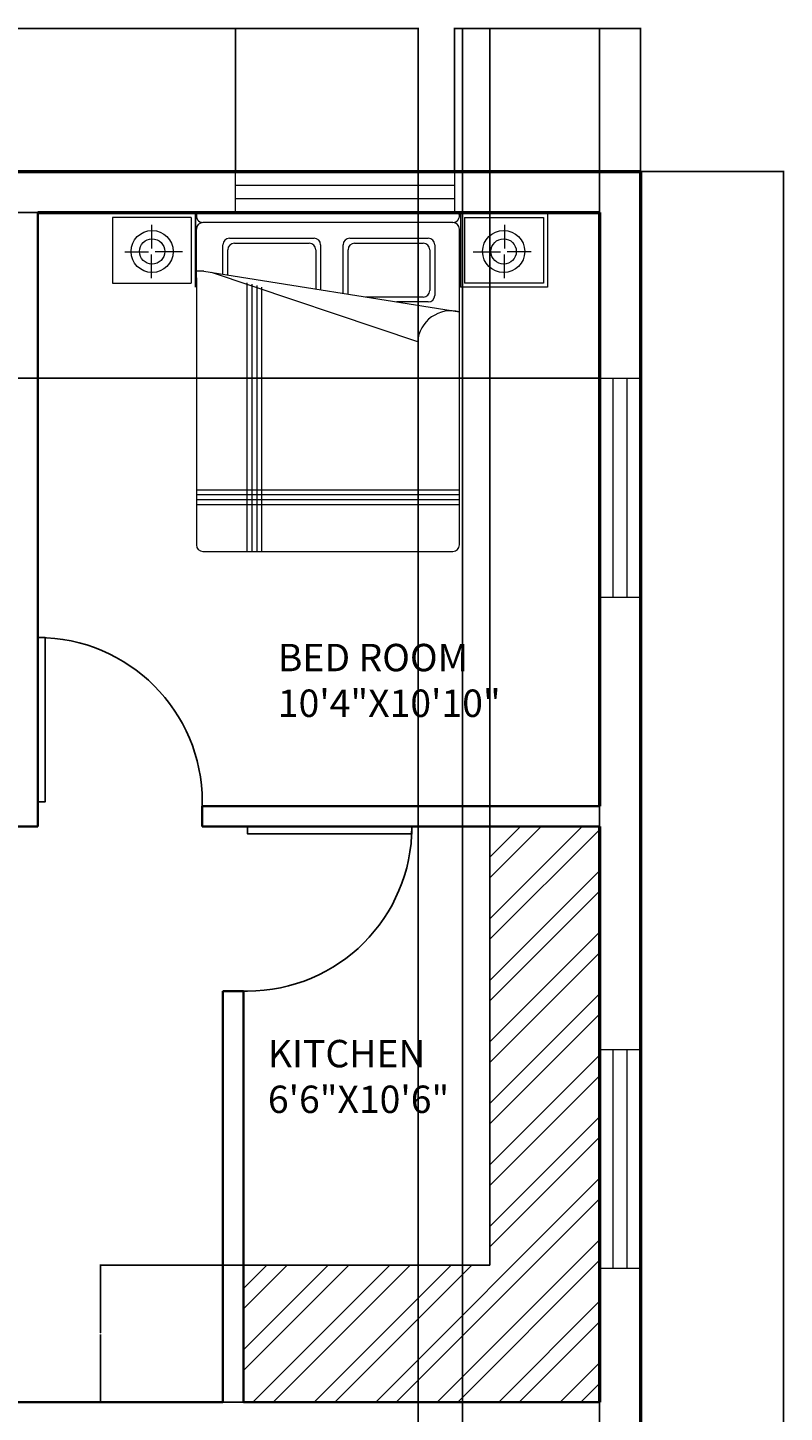
# Model space of a CAD drawing. Units: feet. Extents: x 2664 to 3060, y 1318 to 2005.
# Tile 5 of 5: x 2894 to 3060, y 1702 to 2005. Entities that reach past the tile are written whole.
import ezdxf

# ---------------------------------------------------------------- set-up
doc = ezdxf.new("R2010")
doc.units = ezdxf.units.FT
for name, color, linetype, lineweight in [('A-ANNO-DIMS', 2, 'Continuous', 18), ('A-AREA-IDEN', 109, 'Continuous', 18), ('A-WALL-EXTR', 130, 'Continuous', 50), ('DOOR', 249, 'Continuous', 25), ('FURNITURE', 240, 'Continuous', 13)]:
    doc.layers.add(name, color=color, linetype=linetype, lineweight=lineweight)
for name, color, linetype, lineweight, true_color in [('A-CASE', 41, 'Continuous', 25, 0xf5dd7a), ('A-CASE-PATT', 152, 'Continuous', 13, 0x2776bb), ('A-GLAZ', 222, 'Continuous', 18, 0xd4008b), ('A-WALL-INTR', 41, 'Continuous', 35, 0xf5dd7a)]:
    doc.layers.add(name, color=color, linetype=linetype, lineweight=lineweight, true_color=true_color)
doc.styles.get("Standard").update_dxf_attribs({"font": 'arial.ttf'})
doc.dimstyles.get("Standard").update_dxf_attribs({"dimtxt": 0.18, "dimasz": 0.18, "dimexe": 0.18, "dimexo": 0.0625, "dimgap": 0.09, "dimtad": 0, "dimtih": 1, "dimtoh": 1, "dimdec": 4, "dimzin": 0, "dimdsep": 46, "dimtxsty": 'Standard', "dimcen": 0.09, "dimadec": 0, "dimazin": 0, "dimtfac": 1, "dimtdec": 4, "dimtofl": 0, "dimtmove": 0, "dimatfit": 3, "dimfxl": 1, "dimtolj": 1, "dimtzin": 0, "dimarcsym": 0})

# ---------------------------------------------------------------- blocks, each defined once
blk = doc.blocks.new('*U2')
for p, q in [((0, 0), (0, -6)), ((40, 0), (40, -6))]:
    blk.add_line(p, q)
blk.add_lwpolyline([(0, 0), (0, 40), (1.75, 40), (1.75, 0)], close=True)
blk.add_arc((0, 0), 40, 0, 90)
blk = doc.blocks.new('BED-DOUBLE-WITH-NIGHTSTANDS')
for p, q in [((-29.54, 0), (-29.54, -16.21)), ((-30.37, -0.95), (-47.65, -0.95)), ((-47.65, -0.95), (-47.65, -15.35)), ((-39.11, -2.58), (-39.11, -7.74)), ((-30.37, -0.95), (-30.37, -15.35)), ((-29.47, -0.05), (-29.47, -16.25)), ((28.27, -0.11), (-29.17, -0.11)), ((26.92, -2.06), (-27.82, -2.06)), ((28.57, -0.05), (47.65, -0.05)), ((28.57, -0.05), (28.57, -16.25)), ((29.47, -0.95), (46.75, -0.95)), ((29.47, -0.95), (29.47, -15.35)), ((38.21, -2.58), (38.21, -7.74)), ((46.75, -0.95), (46.75, -15.35)), ((47.65, -0.05), (47.65, -16.25)), ((-29.26, -14.16), (-29.26, -3.5)), ((-22.01, -5.5), (-3.48, -5.5)), ((4.33, -5.5), (21.52, -5.5)), ((28.36, -72.65), (28.36, -3.5)), ((-44.95, -8.46), (-39.75, -8.46)), ((-39.11, -14.22), (-39.11, -9.06)), ((-32.27, -8.46), (-38.27, -8.46)), ((-23.45, -13.32), (-23.45, -6.94)), ((-22.37, -13.47), (-22.37, -8.02)), ((-20.93, -6.58), (-4.56, -6.58)), ((-3.12, -8.02), (-3.12, -16.63)), ((-2.04, -6.94), (-2.04, -16.8)), ((2.88, -17.58), (2.88, -6.94)), ((3.96, -17.76), (3.96, -8.02)), ((5.41, -6.58), (20.44, -6.58)), ((21.88, -8.02), (21.88, -16.94)), ((22.96, -6.94), (22.96, -18.02)), ((31.37, -8.46), (37.37, -8.46)), ((38.21, -14.22), (38.21, -9.06)), ((44.05, -8.46), (38.85, -8.46)), ((-27.62, -12.73), (-29.26, -12.73)), ((-29.26, -14.16), (-29.26, -72.65)), ((-27.62, -12.73), (28.36, -21.64)), ((-26, -12.96), (19.2, -28.15)), ((-47.65, -15.35), (-30.37, -15.35)), ((-18.14, -74.09), (-18.14, -15.24)), ((-17.06, -74.09), (-17.06, -15.55)), ((-15.97, -74.09), (-15.97, -15.86)), ((-14.89, -74.09), (-14.89, -16.18)), ((47.65, -16.25), (28.57, -16.25)), ((46.75, -15.35), (29.47, -15.35)), ((20.44, -18.38), (7.87, -18.38)), ((21.52, -19.46), (14.66, -19.46)), ((28.36, -60.64), (-29.26, -60.64)), ((28.36, -61.72), (-29.26, -61.72)), ((28.36, -62.8), (-29.26, -62.8)), ((28.36, -63.88), (-29.26, -63.88)), ((-27.82, -74.09), (26.92, -74.09))]:
    blk.add_line(p, q)
for centre, radius in [((-38.95, -8.4), 4.61), ((-38.95, -8.4), 2.77), ((38.05, -8.4), 4.61), ((38.05, -8.4), 2.77)]:
    blk.add_circle(centre, radius)
for centre, radius, start, end in [((-27.82, -0.62), 1.44, 159.2884, 270), ((-27.82, -3.5), 1.44, 90, 180), ((26.92, -0.62), 1.44, 270, 20.7116), ((26.92, -3.5), 1.44, 0, 90), ((-22.01, -6.94), 1.44, 90, 180), ((-3.48, -6.94), 1.44, 0, 90), ((4.33, -6.94), 1.44, 90, 180), ((21.52, -6.94), 1.44, 0, 90), ((-20.93, -8.02), 1.44, 90, 180), ((-4.56, -8.02), 1.44, 0, 90), ((5.41, -8.02), 1.44, 90, 180), ((20.44, -8.02), 1.44, 0, 90), ((20.44, -16.94), 1.44, 270, 0), ((21.52, -18.02), 1.44, 270, 0), ((26.5, -28.71), 7.32, 75.237, 175.5647), ((-27.82, -72.65), 1.44, 180, 270), ((26.92, -72.65), 1.44, 270, 0)]:
    blk.add_arc(centre, radius, start, end)
blk = doc.blocks.new('WINDOW-4FT')
for p, q in [((-24, 4.5), (24, 4.5)), ((-24, -4.5), (-24, 4.5)), ((24, 4.5), (24, -4.5)), ((-24, 1.5), (24, 1.5)), ((24, -1.5), (-24, -1.5)), ((24, -4.5), (-24, -4.5))]:
    blk.add_line(p, q)
blk = doc.blocks.new('*D33')
at = {"layer": 'A-ANNO-DIMS', "color": 0, "lineweight": -2, "transparency": 16777216}
for p, q in [((3028.34, 1973.57), (3059.74, 1973.57)), ((3059.56, 1973.39), (3059.56, 1661.75)), ((3059.56, 1349.75), (3059.56, 1661.39)), ((3028.34, 1349.57), (3059.74, 1349.57))]:
    blk.add_line(p, q, dxfattribs=at)
at = {"layer": 'A-ANNO-DIMS', "color": 0, "transparency": 16777216}
for points in [[(3059.53, 1973.39), (3059.59, 1973.39), (3059.56, 1973.57)], [(3059.53, 1349.75), (3059.59, 1349.75), (3059.56, 1349.57)]]:
    blk.add_solid(points, dxfattribs=at)
at = {"layer": 'Defpoints', "color": 0, "transparency": 16777216}
for p in [(3028.28, 1973.57), (3059.56, 1973.57), (3028.28, 1349.57)]:
    blk.add_point(p, dxfattribs=at)
at = {"layer": 'A-ANNO-DIMS', "color": 0, "transparency": 16777216, "insert": (3059.56, 1661.57), "char_height": 0.18, "attachment_point": 5}
blk.add_mtext('\\A1;624', dxfattribs=at)
blk = doc.blocks.new('*D38')
at = {"layer": 'A-ANNO-DIMS', "color": 0, "lineweight": -2, "transparency": 16777216}
for p, q in [((2875.93, 1973.63), (2875.93, 2005.03)), ((2876.11, 2004.85), (2907.35, 2004.85)), ((2939.35, 2004.85), (2908.11, 2004.85)), ((2939.53, 1973.63), (2939.53, 2005.03))]:
    blk.add_line(p, q, dxfattribs=at)
at = {"layer": 'A-ANNO-DIMS', "color": 0, "transparency": 16777216}
for points in [[(2876.11, 2004.88), (2876.11, 2004.82), (2875.93, 2004.85)], [(2939.35, 2004.88), (2939.35, 2004.82), (2939.53, 2004.85)]]:
    blk.add_solid(points, dxfattribs=at)
at = {"layer": 'Defpoints', "color": 0, "transparency": 16777216}
for p in [(2939.53, 2004.85), (2875.93, 1973.57), (2939.53, 1973.57)]:
    blk.add_point(p, dxfattribs=at)
at = {"layer": 'A-ANNO-DIMS', "color": 0, "transparency": 16777216, "insert": (2907.73, 2004.85), "char_height": 0.18, "attachment_point": 5}
blk.add_mtext('\\A1;63.61', dxfattribs=at)
blk = doc.blocks.new('*D39')
at = {"layer": 'A-ANNO-DIMS', "color": 0, "lineweight": -2, "transparency": 16777216}
for p, q in [((2987.53, 1973.63), (2987.53, 2005.03)), ((2987.71, 2004.85), (3007.51, 2004.85)), ((3028.1, 2004.85), (3008.31, 2004.85)), ((3028.28, 1973.63), (3028.28, 2005.03))]:
    blk.add_line(p, q, dxfattribs=at)
at = {"layer": 'A-ANNO-DIMS', "color": 0, "transparency": 16777216}
for points in [[(2987.71, 2004.88), (2987.71, 2004.82), (2987.53, 2004.85)], [(3028.1, 2004.88), (3028.1, 2004.82), (3028.28, 2004.85)]]:
    blk.add_solid(points, dxfattribs=at)
at = {"layer": 'Defpoints', "color": 0, "transparency": 16777216}
for p in [(3028.28, 2004.85), (2987.53, 1973.57), (3028.28, 1973.57)]:
    blk.add_point(p, dxfattribs=at)
at = {"layer": 'A-ANNO-DIMS', "color": 0, "transparency": 16777216, "insert": (3007.91, 2004.85), "char_height": 0.18, "attachment_point": 5}
blk.add_mtext('\\A1;40.75', dxfattribs=at)
blk = doc.blocks.new('*D47')
at = {"layer": 'A-ANNO-DIMS', "color": 0, "lineweight": -2, "transparency": 16777216}
for p, q in [((3019.22, 1964.57), (2663.82, 1964.57)), ((2664, 1964.39), (2664, 1946.59)), ((2664, 1928.43), (2664, 1946.23)), ((3019.22, 1928.25), (2663.82, 1928.25))]:
    blk.add_line(p, q, dxfattribs=at)
at = {"layer": 'A-ANNO-DIMS', "color": 0, "transparency": 16777216}
for points in [[(2663.97, 1964.39), (2664.03, 1964.39), (2664, 1964.57)], [(2663.97, 1928.43), (2664.03, 1928.43), (2664, 1928.25)]]:
    blk.add_solid(points, dxfattribs=at)
at = {"layer": 'Defpoints', "color": 0, "transparency": 16777216}
for p in [(3019.28, 1964.57), (2664, 1928.25), (3019.28, 1928.25)]:
    blk.add_point(p, dxfattribs=at)
at = {"layer": 'A-ANNO-DIMS', "color": 0, "transparency": 16777216, "insert": (2664, 1946.41), "char_height": 0.18, "attachment_point": 5}
blk.add_mtext('\\A1;36.32', dxfattribs=at)
blk = doc.blocks.new('*D48')
at = {"layer": 'A-ANNO-DIMS', "color": 0, "lineweight": -2, "transparency": 16777216}
for p, q in [((2879.53, 1619.63), (2879.53, 2005.03)), ((2879.71, 2004.85), (2929.25, 2004.85)), ((2979.35, 2004.85), (2929.81, 2004.85)), ((2979.53, 1619.63), (2979.53, 2005.03))]:
    blk.add_line(p, q, dxfattribs=at)
at = {"layer": 'A-ANNO-DIMS', "color": 0, "transparency": 16777216}
for points in [[(2879.71, 2004.88), (2879.71, 2004.82), (2879.53, 2004.85)], [(2979.35, 2004.88), (2979.35, 2004.82), (2979.53, 2004.85)]]:
    blk.add_solid(points, dxfattribs=at)
at = {"layer": 'Defpoints', "color": 0, "transparency": 16777216}
for p in [(2979.53, 2004.85), (2879.53, 1619.57), (2979.53, 1619.57)]:
    blk.add_point(p, dxfattribs=at)
at = {"layer": 'A-ANNO-DIMS', "color": 0, "transparency": 16777216, "insert": (2929.53, 2004.85), "char_height": 0.18, "attachment_point": 5}
blk.add_mtext('\\A1;100', dxfattribs=at)
blk = doc.blocks.new('*D56')
at = {"layer": 'A-ANNO-DIMS', "color": 0, "lineweight": -2, "transparency": 16777216}
for p, q in [((2995.28, 1830.13), (2995.28, 2005.03)), ((2995.46, 2004.85), (3007.06, 2004.85)), ((3019.1, 2004.85), (3007.5, 2004.85)), ((3019.28, 1830.13), (3019.28, 2005.03))]:
    blk.add_line(p, q, dxfattribs=at)
at = {"layer": 'A-ANNO-DIMS', "color": 0, "transparency": 16777216}
for points in [[(2995.46, 2004.88), (2995.46, 2004.82), (2995.28, 2004.85)], [(3019.1, 2004.88), (3019.1, 2004.82), (3019.28, 2004.85)]]:
    blk.add_solid(points, dxfattribs=at)
at = {"layer": 'Defpoints', "color": 0, "transparency": 16777216}
for p in [(3019.28, 2004.85), (2995.28, 1830.07), (3019.28, 1830.07)]:
    blk.add_point(p, dxfattribs=at)
at = {"layer": 'A-ANNO-DIMS', "color": 0, "transparency": 16777216, "insert": (3007.28, 2004.85), "char_height": 0.18, "attachment_point": 5}
blk.add_mtext('\\A1;24', dxfattribs=at)
blk = doc.blocks.new('*D57')
at = {"layer": 'A-ANNO-DIMS', "color": 0, "lineweight": -2, "transparency": 16777216}
for p, q in [((2941.22, 1734.07), (2909.82, 1734.07)), ((2910, 1733.89), (2910, 1719.25)), ((2910, 1704.25), (2910, 1718.89)), ((2941.22, 1704.07), (2909.82, 1704.07))]:
    blk.add_line(p, q, dxfattribs=at)
at = {"layer": 'A-ANNO-DIMS', "color": 0, "transparency": 16777216}
for points in [[(2909.97, 1733.89), (2910.03, 1733.89), (2910, 1734.07)], [(2909.97, 1704.25), (2910.03, 1704.25), (2910, 1704.07)]]:
    blk.add_solid(points, dxfattribs=at)
at = {"layer": 'Defpoints', "color": 0, "transparency": 16777216}
for p in [(2910, 1734.07), (2941.28, 1734.07), (2941.28, 1704.07)]:
    blk.add_point(p, dxfattribs=at)
at = {"layer": 'A-ANNO-DIMS', "color": 0, "transparency": 16777216, "insert": (2910, 1719.07), "char_height": 0.18, "attachment_point": 5}
blk.add_mtext('\\A1;30', dxfattribs=at)
blk = doc.blocks.new('*D58')
at = {"layer": 'A-ANNO-DIMS', "color": 0, "lineweight": -2, "transparency": 16777216}
for p, q in [((2989.28, 1488.63), (2989.28, 2005.03)), ((2989.46, 2004.85), (3004.06, 2004.85)), ((3019.1, 2004.85), (3004.5, 2004.85)), ((3019.28, 1488.63), (3019.28, 2005.03))]:
    blk.add_line(p, q, dxfattribs=at)
at = {"layer": 'A-ANNO-DIMS', "color": 0, "transparency": 16777216}
for points in [[(2989.46, 2004.88), (2989.46, 2004.82), (2989.28, 2004.85)], [(3019.1, 2004.88), (3019.1, 2004.82), (3019.28, 2004.85)]]:
    blk.add_solid(points, dxfattribs=at)
at = {"layer": 'Defpoints', "color": 0, "transparency": 16777216}
for p in [(3019.28, 2004.85), (2989.28, 1488.57), (3019.28, 1488.57)]:
    blk.add_point(p, dxfattribs=at)
at = {"layer": 'A-ANNO-DIMS', "color": 0, "transparency": 16777216, "insert": (3004.28, 2004.85), "char_height": 0.18, "attachment_point": 5}
blk.add_mtext('\\A1;30', dxfattribs=at)

msp = doc.modelspace()

# ---------------------------------------------------------------- hatches: boundary and pattern name
at = {"layer": 'A-CASE-PATT'}
h = msp.add_hatch(dxfattribs=at)
h.set_pattern_fill('ANSI32', color=256)
h.paths.add_polyline_path([(3019.28, 1615.071), (2941.28, 1615.071), (2941.28, 1585.071), (2989.28, 1585.071), (2989.28, 1488.571), (3019.28, 1488.571)])
h.paths.add_polyline_path([(3019.28, 1830.071), (2995.28, 1830.071), (2995.28, 1734.071), (2941.28, 1734.071), (2941.28, 1704.071), (3019.28, 1704.071)])

# ---------------------------------------------------------------- linework, layer by layer
at = {"layer": 'A-CASE'}
for p in [(2995.28, 1830.071), (2941.28, 1734.071)]:
    msp.add_line(p, (2995.28, 1734.071), dxfattribs=at)
at = {"layer": 'A-WALL-EXTR'}
for p, q in [((2704.28, 1973.571), (3028.28, 1973.571)), ((3028.28, 1973.571), (3028.28, 1349.571)), ((2896.28, 1964.571), (3019.28, 1964.571)), ((3019.28, 1964.571), (3019.28, 1834.571)), ((3019.28, 1830.071), (3019.28, 1704.071))]:
    msp.add_line(p, q, dxfattribs=at)
at = {"layer": 'A-WALL-INTR'}
for p, q in [((2896.28, 1834.571), (2896.28, 1964.571)), ((2896.28, 1834.571), (2896.28, 1830.071)), ((2932.28, 1834.571), (3019.28, 1834.571)), ((2932.28, 1834.571), (2932.28, 1830.071)), ((2891.78, 1830.071), (2896.28, 1830.071)), ((2932.28, 1830.071), (2936.78, 1830.071)), ((2936.78, 1830.071), (2941.28, 1830.071)), ((2941.28, 1830.071), (3019.28, 1830.071)), ((2936.78, 1794.071), (2936.78, 1704.071)), ((2936.78, 1794.071), (2941.28, 1794.071)), ((2941.28, 1794.071), (2941.28, 1704.071)), ((2866.78, 1704.071), (2936.78, 1704.071)), ((2941.28, 1704.071), (3019.28, 1704.071))]:
    msp.add_line(p, q, dxfattribs=at)

# ---------------------------------------------------------------- block references
at = {"layer": 'A-GLAZ'}
for p, rotation in [((2963.534, 1969.071), 180), ((3023.78, 1904.253), 89.99999999999844), ((3023.78, 1757.306), 89.99999999999864)]:
    msp.add_blockref('WINDOW-4FT', p, dxfattribs=dict(at, rotation=rotation))
at = {"layer": 'DOOR', "xscale": 0.899999999999959, "yscale": 0.899999999999959, "zscale": 0.899999999999959}
msp.add_blockref('*U2', (2896.28, 1835.471), dxfattribs=at)
at = {"layer": 'DOOR', "xscale": 0.899999999999959, "yscale": 0.899999999999959, "zscale": 0.899999999999959, "rotation": 270}
msp.add_blockref('*U2', (2942.18, 1830.071), dxfattribs=at)
at = {"layer": 'FURNITURE'}
msp.add_blockref('BED-DOUBLE-WITH-NIGHTSTANDS', (2960.234, 1964.426), dxfattribs=at)

# ---------------------------------------------------------------- texts
at = {"layer": 'A-AREA-IDEN', "char_height": 6, "attachment_point": 1}
for s, width, insert in [('BED ROOM \\P10\'4"X10\'10"', 48.82765, (2948.825, 1870.1)), ('KITCHEN\\P6\'6"X10\'6"', 22.955, (2946.648, 1783.368))]:
    msp.add_mtext_dynamic_manual_height_columns(s, width=width, gutter_width=12.5, heights=[0], dxfattribs=dict(at, insert=insert))

# ---------------------------------------------------------------- dimensions: what is measured, and where the dimension line sits
at = {"layer": 'A-ANNO-DIMS'}
for base, p1, p2, override, picture, middle in [((2939.534, 2004.851), (2875.926, 1973.571), (2939.534, 1973.571), {"dimdec": 2, "dimlfac": 1, "dimrnd": 0, "dimzin": 0, "dimdsep": 46, "dimlunit": 2}, '*D38', (2907.73, 2004.851)), ((2979.53, 2004.851), (2879.53, 1619.571), (2979.53, 1619.571), {"dimdec": 0, "dimlfac": 1, "dimrnd": 0, "dimzin": 0, "dimdsep": 46, "dimlunit": 2}, '*D48', (2929.53, 2004.851)), ((3028.28, 2004.851), (2987.534, 1973.571), (3028.28, 1973.571), {"dimdec": 2, "dimlfac": 1, "dimrnd": 0, "dimzin": 0, "dimdsep": 46, "dimlunit": 2}, '*D39', (3007.907, 2004.851)), ((3019.28, 2004.851), (2989.28, 1488.571), (3019.28, 1488.571), {"dimdec": 0, "dimlfac": 1, "dimrnd": 0, "dimzin": 0, "dimdsep": 46, "dimlunit": 2}, '*D58', (3004.28, 2004.851)), ((3019.28, 2004.851), (2995.28, 1830.071), (3019.28, 1830.071), {"dimdec": 0, "dimlfac": 1, "dimrnd": 0, "dimzin": 0, "dimdsep": 46, "dimlunit": 2}, '*D56', (3007.28, 2004.851))]:
    dim = msp.add_linear_dim(base=base, p1=p1, p2=p2, dimstyle='Standard', override=override, dxfattribs=at)
    dim.commit()
    dim.dimension.update_dxf_attribs({"geometry": picture, "text_midpoint": middle})
for base, p1, p2, override, picture, middle in [((3059.56, 1973.571), (3028.28, 1349.571), (3028.28, 1973.571), {"dimdec": 0, "dimlfac": 1, "dimrnd": 0, "dimzin": 0, "dimdsep": 46, "dimlunit": 2}, '*D33', (3059.56, 1661.571)), ((2664, 1928.253), (3019.28, 1964.571), (3019.28, 1928.253), {"dimdec": 2, "dimlfac": 1, "dimrnd": 0, "dimzin": 0, "dimdsep": 46, "dimlunit": 2}, '*D47', (2664, 1946.412)), ((2910, 1734.071), (2941.28, 1704.071), (2941.28, 1734.071), {"dimdec": 0, "dimlfac": 1, "dimrnd": 0, "dimzin": 0, "dimdsep": 46, "dimlunit": 2}, '*D57', (2910, 1719.071))]:
    dim = msp.add_linear_dim(base=base, p1=p1, p2=p2, angle=90, dimstyle='Standard', override=override, dxfattribs=at)
    dim.commit()
    dim.dimension.update_dxf_attribs({"geometry": picture, "text_midpoint": middle})

doc.saveas('drawing.dxf')
